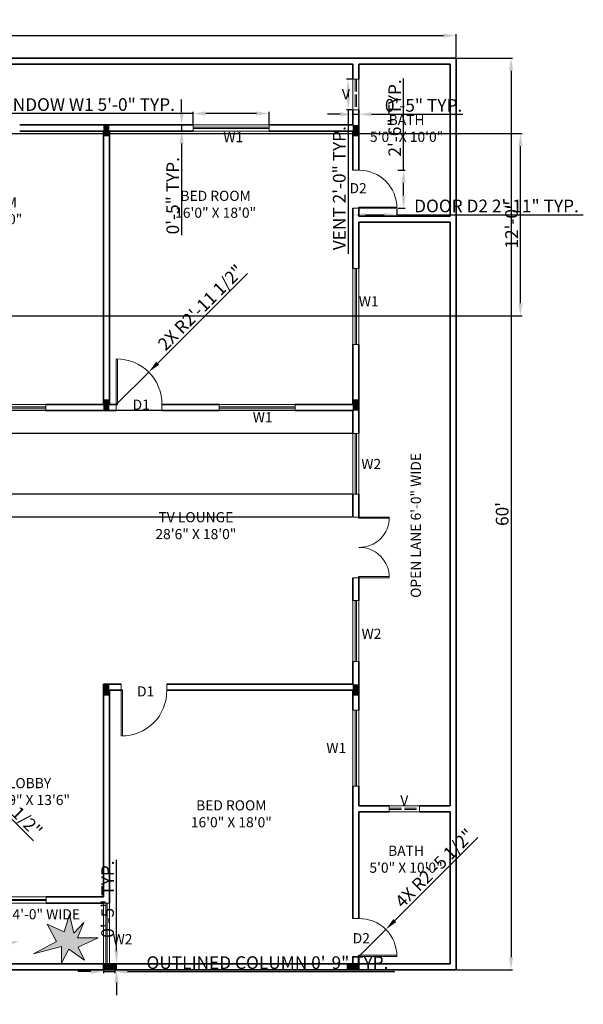
# Model space of a CAD drawing. Units: inches. Extents: x 13878 to 15021, y 3891 to 4810.
# Tile 3 of 3: x 14576 to 15021, y 3923 to 4701. Entities that reach past the tile are written whole.
import ezdxf

# ---------------------------------------------------------------- set-up
doc = ezdxf.new("R2010")
doc.units = ezdxf.units.IN
doc.linetypes.add('ACAD_ISO02W100', pattern=[15, 12, -3])
for name, color, linetype, lineweight in [('A-ANNO-DIMS', 2, 'Continuous', 18), ('A-ANNO-TEXT', 7, 'Continuous', 18), ('A-AREA-IDEN', 7, 'Continuous', 18), ('A-COLS', 7, 'Continuous', 35), ('A-COLS-PATT', 7, 'Continuous', 18), ('A-DOOR', 4, 'Continuous', 18), ('A-GLAZ', 4, 'Continuous', 18), ('A-GLAZ-HIDN', 4, 'ACAD_ISO02W100', 13), ('A-WALL', 150, 'Continuous', 35), ('C-SITE-WALL', 150, 'Continuous', 35), ('L-PLNT', 85, 'Continuous', 18)]:
    doc.layers.add(name, color=color, linetype=linetype, lineweight=lineweight)
doc.layers.add('L-PLNT-PATT', color=85, linetype='Continuous', lineweight=13, true_color=0x58ba48)
doc.styles.get("Standard").update_dxf_attribs({"font": 'arial.ttf'})
doc.dimstyles.new('ISO-25', dxfattribs={"dimtxt": 10, "dimasz": 10, "dimexe": 1.25, "dimexo": 0.625, "dimtad": 1, "dimdec": 0, "dimlunit": 3, "dimtxsty": 'Standard', "dimcen": 2.5, "dimadec": 0, "dimazin": 0, "dimtfac": 1, "dimtdec": 0, "dimtmove": 0, "dimatfit": 3, "dimfxl": 1, "dimarcsym": 0})

# ---------------------------------------------------------------- blocks, each defined once
blk = doc.blocks.new('*D7')
at = {"layer": 'A-ANNO-DIMS', "color": 0, "lineweight": -2, "transparency": 16777216}
for p, q in [((13960.64, 4671.28), (13960.64, 4689.65)), ((13970.64, 4688.4), (14910.64, 4688.4)), ((14920.64, 4671.28), (14920.64, 4689.65))]:
    blk.add_line(p, q, dxfattribs=at)
at = {"layer": 'A-ANNO-DIMS', "color": 0, "transparency": 16777216}
for points in [[(13970.64, 4690.07), (13970.64, 4686.74), (13960.64, 4688.4)], [(14910.64, 4690.07), (14910.64, 4686.74), (14920.64, 4688.4)]]:
    blk.add_solid(points, dxfattribs=at)
at = {"layer": 'Defpoints', "color": 0, "transparency": 16777216}
for p in [(14920.64, 4688.4), (13960.64, 4670.66), (14920.64, 4670.66)]:
    blk.add_point(p, dxfattribs=at)
at = {"layer": 'A-ANNO-DIMS', "color": 0, "transparency": 16777216, "insert": (14440.64, 4694.14), "char_height": 10, "attachment_point": 5}
blk.add_mtext("80'", dxfattribs=at)
blk = doc.blocks.new('*D8')
at = {"layer": 'A-ANNO-DIMS', "color": 0, "lineweight": -2, "transparency": 16777216}
for p, q in [((14921.26, 4670.66), (14965.22, 4670.66)), ((14963.97, 4660.66), (14963.97, 3960.66)), ((14921.26, 3950.66), (14965.22, 3950.66))]:
    blk.add_line(p, q, dxfattribs=at)
at = {"layer": 'A-ANNO-DIMS', "color": 0, "transparency": 16777216}
for points in [[(14962.31, 4660.66), (14965.64, 4660.66), (14963.97, 4670.66)], [(14962.31, 3960.66), (14965.64, 3960.66), (14963.97, 3950.66)]]:
    blk.add_solid(points, dxfattribs=at)
at = {"layer": 'Defpoints', "color": 0, "transparency": 16777216}
for p in [(14920.64, 4670.66), (14920.64, 3950.66), (14963.97, 3950.66)]:
    blk.add_point(p, dxfattribs=at)
at = {"layer": 'A-ANNO-DIMS', "color": 0, "transparency": 16777216, "insert": (14958.24, 4310.66), "char_height": 10, "attachment_point": 5, "rotation": 90}
blk.add_mtext("60'", dxfattribs=at)
blk = doc.blocks.new('DOOR-D1-36IN')
for p, q in [((0, 4.8), (0, 40.8)), ((1, 4.8), (1, 40.8)), ((0, 4.8), (0, 0)), ((36, 4.8), (36, 0))]:
    blk.add_line(p, q)
blk.add_arc((0.5, 5.3), 35.5, 359.19307, 90.80693)
blk = doc.blocks.new('DOOR-D2-30IN')
for p, q in [((0, 30), (4.8, 30)), ((0, 0), (4.8, 0)), ((4.8, 1), (34.8, 1)), ((4.8, 0), (34.8, 0))]:
    blk.add_line(p, q)
blk.add_arc((5.3, 0.5), 29.5, 359.02898, 90.97102)
blk = doc.blocks.new('DOOR-PAIR-48IN')
for p, q in [((0, 48), (4.8, 48)), ((4.8, 48), (28.8, 48)), ((4.8, 47), (28.8, 47)), ((4.8, 1), (28.8, 1)), ((0, 0), (4.8, 0)), ((4.8, 0), (28.8, 0))]:
    blk.add_line(p, q)
for centre, start, end in [((5.3, 47.5), 268.78112, 1.21888), ((5.3, 0.5), 358.78112, 91.21888)]:
    blk.add_arc(centre, 23.51, start, end)
blk = doc.blocks.new('WINDOW-W1-60IN')
for p, q in [((0, 0), (0, 4.8)), ((0, 4.8), (60, 4.8)), ((0, 2.9), (60, 2.9)), ((0, 1.9), (60, 1.9)), ((60, 0), (60, 4.8)), ((0, 0), (60, 0))]:
    blk.add_line(p, q)
blk = doc.blocks.new('WINDOW-W2-48IN')
for p, q in [((0, 0), (0, 4.8)), ((0, 4.8), (48, 4.8)), ((0, 2.9), (48, 2.9)), ((0, 1.9), (48, 1.9)), ((48, 0), (48, 4.8)), ((0, 0), (48, 0))]:
    blk.add_line(p, q)
blk = doc.blocks.new('COLUMN-RECT-OUTLINED')
h = blk.add_hatch(color=256)
h.dxf.hatch_style = 1
h.paths.add_polyline_path([(9, 0), (9, 4.8), (0, 4.8), (0, 0)])
for p, q in [((0, 4.8), (0, 0)), ((9, 4.8), (0, 4.8)), ((9, 0), (9, 4.8)), ((0, 0), (9, 0))]:
    blk.add_line(p, q)
blk = doc.blocks.new('COLUMN-RECT-SOLID')
h = blk.add_hatch(color=256)
h.dxf.hatch_style = 1
h.paths.add_polyline_path([(0, 0), (4.8, 0), (4.8, 9), (0, 9)])
blk = doc.blocks.new('VENT-FRAME-24IN')
for p, q in [((0, 0), (0, 4.8)), ((0, 4.8), (24, 4.8)), ((24, 0), (24, 4.8)), ((0, 0), (24, 0))]:
    blk.add_line(p, q)
blk = doc.blocks.new('*D20')
at = {"layer": 'A-ANNO-DIMS', "color": 0, "lineweight": -2, "ltscale": 2, "transparency": 16777216}
for p, q in [((14642.24, 3950.03), (14642.24, 3948.06)), ((14651.24, 3950.03), (14651.24, 3948.06)), ((14632.24, 3949.31), (14622.24, 3949.31)), ((14642.24, 3949.31), (14651.24, 3949.31)), ((14661.24, 3949.31), (14872.28, 3949.31))]:
    blk.add_line(p, q, dxfattribs=at)
at = {"layer": 'A-ANNO-DIMS', "color": 0, "ltscale": 2, "transparency": 16777216}
for points in [[(14632.24, 3950.98), (14632.24, 3947.64), (14642.24, 3949.31)], [(14661.24, 3950.98), (14661.24, 3947.64), (14651.24, 3949.31)]]:
    blk.add_solid(points, dxfattribs=at)
at = {"layer": 'Defpoints', "color": 0, "ltscale": 2, "transparency": 16777216}
for p in [(14642.24, 3950.66), (14651.24, 3950.66), (14651.24, 3949.31)]:
    blk.add_point(p, dxfattribs=at)
at = {"layer": 'A-ANNO-DIMS', "color": 0, "ltscale": 2, "transparency": 16777216, "insert": (14771.76, 3955.11), "char_height": 10, "attachment_point": 5}
blk.add_mtext('OUTLINED COLUMN 0\'-9" TYP.', dxfattribs=at)
blk = doc.blocks.new('*D21')
at = {"layer": 'A-ANNO-DIMS', "color": 0, "lineweight": -2, "ltscale": 2, "transparency": 16777216}
for p, q in [((14652.59, 3965.46), (14652.59, 4037.66)), ((14651.86, 3955.46), (14653.84, 3955.46)), ((14651.86, 3950.66), (14653.84, 3950.66)), ((14652.59, 3950.66), (14652.59, 3955.46)), ((14652.59, 3940.66), (14652.59, 3930.66))]:
    blk.add_line(p, q, dxfattribs=at)
at = {"layer": 'A-ANNO-DIMS', "color": 0, "ltscale": 2, "transparency": 16777216}
for points in [[(14650.92, 3965.46), (14654.25, 3965.46), (14652.59, 3955.46)], [(14650.92, 3940.66), (14654.25, 3940.66), (14652.59, 3950.66)]]:
    blk.add_solid(points, dxfattribs=at)
at = {"layer": 'Defpoints', "color": 0, "ltscale": 2, "transparency": 16777216}
for p in [(14651.24, 3955.46), (14651.24, 3950.66), (14652.59, 3955.46)]:
    blk.add_point(p, dxfattribs=at)
at = {"layer": 'A-ANNO-DIMS', "color": 0, "ltscale": 2, "transparency": 16777216, "insert": (14646.86, 4006.56), "char_height": 10, "attachment_point": 5, "rotation": 90}
blk.add_mtext('0\'-5" TYP.', dxfattribs=at)
blk = doc.blocks.new('*D24')
at = {"layer": 'A-ANNO-DIMS', "color": 0, "lineweight": -2, "ltscale": 2, "transparency": 16777216}
for p, q in [((14713.04, 4626.86), (14550.41, 4626.86)), ((14713.04, 4618.48), (14713.04, 4628.11)), ((14763.04, 4626.86), (14723.04, 4626.86)), ((14773.04, 4618.48), (14773.04, 4628.11))]:
    blk.add_line(p, q, dxfattribs=at)
at = {"layer": 'A-ANNO-DIMS', "color": 0, "ltscale": 2, "transparency": 16777216}
for points in [[(14723.04, 4628.53), (14723.04, 4625.19), (14713.04, 4626.86)], [(14763.04, 4628.53), (14763.04, 4625.19), (14773.04, 4626.86)]]:
    blk.add_solid(points, dxfattribs=at)
at = {"layer": 'Defpoints', "color": 0, "ltscale": 2, "transparency": 16777216}
for p in [(14713.04, 4626.86), (14713.04, 4617.86), (14773.04, 4617.86)]:
    blk.add_point(p, dxfattribs=at)
at = {"layer": 'A-ANNO-DIMS', "color": 0, "ltscale": 2, "transparency": 16777216, "insert": (14626.72, 4632.66), "char_height": 10, "attachment_point": 5}
blk.add_mtext('WINDOW W1 5\'-0" TYP.', dxfattribs=at)
blk = doc.blocks.new('*D25')
at = {"layer": 'A-ANNO-DIMS', "color": 0, "lineweight": -2, "ltscale": 2, "transparency": 16777216}
for p, q in [((14704.04, 4627.86), (14704.04, 4637.86)), ((14712.41, 4617.86), (14702.79, 4617.86)), ((14712.41, 4613.06), (14702.79, 4613.06)), ((14704.04, 4617.86), (14704.04, 4613.06)), ((14704.04, 4603.06), (14704.04, 4530.85))]:
    blk.add_line(p, q, dxfattribs=at)
at = {"layer": 'A-ANNO-DIMS', "color": 0, "ltscale": 2, "transparency": 16777216}
for points in [[(14702.37, 4627.86), (14705.7, 4627.86), (14704.04, 4617.86)], [(14702.37, 4603.06), (14705.7, 4603.06), (14704.04, 4613.06)]]:
    blk.add_solid(points, dxfattribs=at)
at = {"layer": 'Defpoints', "color": 0, "ltscale": 2, "transparency": 16777216}
for p in [(14704.04, 4613.06), (14713.04, 4617.86), (14713.04, 4613.06)]:
    blk.add_point(p, dxfattribs=at)
at = {"layer": 'A-ANNO-DIMS', "color": 0, "ltscale": 2, "transparency": 16777216, "insert": (14698.31, 4561.96), "char_height": 10, "attachment_point": 5, "rotation": 90}
blk.add_mtext('0\'-5" TYP.', dxfattribs=at)
blk = doc.blocks.new('*D28')
at = {"layer": 'A-ANNO-DIMS', "color": 0, "lineweight": -2, "ltscale": 2, "transparency": 16777216}
for p, q in [((14838.41, 4653.86), (14834.19, 4653.86)), ((14835.44, 4643.86), (14835.44, 4639.86)), ((14838.41, 4629.86), (14834.19, 4629.86)), ((14835.44, 4629.86), (14835.44, 4516))]:
    blk.add_line(p, q, dxfattribs=at)
at = {"layer": 'A-ANNO-DIMS', "color": 0, "ltscale": 2, "transparency": 16777216}
for points in [[(14833.77, 4643.86), (14837.1, 4643.86), (14835.44, 4653.86)], [(14833.77, 4639.86), (14837.1, 4639.86), (14835.44, 4629.86)]]:
    blk.add_solid(points, dxfattribs=at)
at = {"layer": 'Defpoints', "color": 0, "ltscale": 2, "transparency": 16777216}
for p in [(14839.04, 4653.86), (14835.44, 4629.86), (14839.04, 4629.86)]:
    blk.add_point(p, dxfattribs=at)
at = {"layer": 'A-ANNO-DIMS', "color": 0, "ltscale": 2, "transparency": 16777216, "insert": (14829.71, 4567.93), "char_height": 10, "attachment_point": 5, "rotation": 90}
blk.add_mtext('VENT 2\'-0" TYP.', dxfattribs=at)
blk = doc.blocks.new('*D29')
at = {"layer": 'A-ANNO-DIMS', "color": 0, "lineweight": -2, "ltscale": 2, "transparency": 16777216}
for p, q in [((14829.04, 4626.26), (14819.04, 4626.26)), ((14839.04, 4629.23), (14839.04, 4625.01)), ((14839.04, 4626.26), (14843.84, 4626.26)), ((14843.84, 4629.23), (14843.84, 4625.01)), ((14853.84, 4626.26), (14926.04, 4626.26))]:
    blk.add_line(p, q, dxfattribs=at)
at = {"layer": 'A-ANNO-DIMS', "color": 0, "ltscale": 2, "transparency": 16777216}
for points in [[(14829.04, 4627.93), (14829.04, 4624.59), (14839.04, 4626.26)], [(14853.84, 4627.93), (14853.84, 4624.59), (14843.84, 4626.26)]]:
    blk.add_solid(points, dxfattribs=at)
at = {"layer": 'Defpoints', "color": 0, "ltscale": 2, "transparency": 16777216}
for p in [(14839.04, 4629.86), (14843.84, 4629.86), (14843.84, 4626.26)]:
    blk.add_point(p, dxfattribs=at)
at = {"layer": 'A-ANNO-DIMS', "color": 0, "ltscale": 2, "transparency": 16777216, "insert": (14894.94, 4631.99), "char_height": 10, "attachment_point": 5}
blk.add_mtext('0\'-5" TYP.', dxfattribs=at)
blk = doc.blocks.new('*D32')
at = {"layer": 'A-ANNO-DIMS', "color": 0, "lineweight": -2, "ltscale": 2, "transparency": 16777216}
for p, q in [((14839.04, 4551.41), (14839.04, 4545.54)), ((14873.97, 4551.41), (14873.97, 4545.54)), ((14849.04, 4546.79), (14863.97, 4546.79)), ((14873.97, 4546.79), (15020.98, 4546.79))]:
    blk.add_line(p, q, dxfattribs=at)
at = {"layer": 'A-ANNO-DIMS', "color": 0, "ltscale": 2, "transparency": 16777216}
for points in [[(14849.04, 4548.46), (14849.04, 4545.13), (14839.04, 4546.79)], [(14863.97, 4548.46), (14863.97, 4545.13), (14873.97, 4546.79)]]:
    blk.add_solid(points, dxfattribs=at)
at = {"layer": 'Defpoints', "color": 0, "ltscale": 2, "transparency": 16777216}
for p in [(14839.04, 4552.03), (14873.97, 4552.03), (14873.97, 4546.79)]:
    blk.add_point(p, dxfattribs=at)
at = {"layer": 'A-ANNO-DIMS', "color": 0, "ltscale": 2, "transparency": 16777216, "insert": (14952.48, 4552.59), "char_height": 10, "attachment_point": 5}
blk.add_mtext('DOOR D2 2\'-11" TYP.', dxfattribs=at)
blk = doc.blocks.new('*D33')
at = {"layer": 'A-ANNO-DIMS', "color": 0, "lineweight": -2, "ltscale": 2, "transparency": 16777216}
for p, q in [((14879.21, 4582.17), (14879.21, 4654.54)), ((14874.6, 4582.17), (14880.46, 4582.17)), ((14879.21, 4562.03), (14879.21, 4572.17)), ((14874.6, 4552.03), (14880.46, 4552.03))]:
    blk.add_line(p, q, dxfattribs=at)
at = {"layer": 'A-ANNO-DIMS', "color": 0, "ltscale": 2, "transparency": 16777216}
for points in [[(14877.55, 4572.17), (14880.88, 4572.17), (14879.21, 4582.17)], [(14877.55, 4562.03), (14880.88, 4562.03), (14879.21, 4552.03)]]:
    blk.add_solid(points, dxfattribs=at)
at = {"layer": 'Defpoints', "color": 0, "ltscale": 2, "transparency": 16777216}
for p in [(14873.97, 4582.17), (14879.21, 4582.17), (14873.97, 4552.03)]:
    blk.add_point(p, dxfattribs=at)
at = {"layer": 'A-ANNO-DIMS', "color": 0, "ltscale": 2, "transparency": 16777216, "insert": (14873.48, 4623.36), "char_height": 10, "attachment_point": 5, "rotation": 90}
blk.add_mtext('2\'-6" TYP.', dxfattribs=at)
blk = doc.blocks.new('*D37')
at = {"layer": 'A-ANNO-DIMS', "color": 0, "lineweight": -2, "ltscale": 2, "transparency": 16777216}
for p, q in [((14030.86, 4611.06), (14972.64, 4611.06)), ((14971.39, 4477.06), (14971.39, 4601.06)), ((14030.86, 4467.06), (14972.64, 4467.06))]:
    blk.add_line(p, q, dxfattribs=at)
at = {"layer": 'A-ANNO-DIMS', "color": 0, "ltscale": 2, "transparency": 16777216}
for points in [[(14969.72, 4601.06), (14973.05, 4601.06), (14971.39, 4611.06)], [(14969.72, 4477.06), (14973.05, 4477.06), (14971.39, 4467.06)]]:
    blk.add_solid(points, dxfattribs=at)
at = {"layer": 'Defpoints', "color": 0, "ltscale": 2, "transparency": 16777216}
for p in [(14030.24, 4611.06), (14971.39, 4611.06), (14030.24, 4467.06)]:
    blk.add_point(p, dxfattribs=at)
at = {"layer": 'A-ANNO-DIMS', "color": 0, "ltscale": 2, "transparency": 16777216, "insert": (14965.66, 4539.06), "char_height": 10, "attachment_point": 5, "rotation": 90}
blk.add_mtext('12\'-0"', dxfattribs=at)
blk = doc.blocks.new('*D40')
at = {"layer": 'A-ANNO-DIMS', "color": 0, "lineweight": -2, "ltscale": 2, "transparency": 16777216}
for p, q in [((13909.89, 4402.26), (13909.89, 4412.26)), ((14838.41, 4392.26), (13908.64, 4392.26)), ((13909.89, 4392.26), (13909.89, 4374.26)), ((14838.41, 4374.26), (13908.64, 4374.26)), ((13909.89, 4364.26), (13909.89, 4327.37))]:
    blk.add_line(p, q, dxfattribs=at)
at = {"layer": 'A-ANNO-DIMS', "color": 0, "ltscale": 2, "transparency": 16777216}
for points in [[(13908.22, 4402.26), (13911.55, 4402.26), (13909.89, 4392.26)], [(13908.22, 4364.26), (13911.55, 4364.26), (13909.89, 4374.26)]]:
    blk.add_solid(points, dxfattribs=at)
at = {"layer": 'Defpoints', "color": 0, "ltscale": 2, "transparency": 16777216}
for p in [(14839.04, 4392.26), (13909.89, 4374.26), (14839.04, 4374.26)]:
    blk.add_point(p, dxfattribs=at)
at = {"layer": 'A-ANNO-DIMS', "color": 0, "ltscale": 2, "transparency": 16777216, "insert": (13904.16, 4340.81), "char_height": 10, "attachment_point": 5, "rotation": 90}
blk.add_mtext('1\'-6"', dxfattribs=at)
blk = doc.blocks.new('*D41')
at = {"layer": 'A-ANNO-DIMS', "color": 0, "lineweight": -2, "ltscale": 2, "transparency": 16777216}
for p, q in [((13909.89, 4336.26), (13909.89, 4346.26)), ((14838.41, 4326.26), (13908.64, 4326.26)), ((13909.89, 4326.26), (13909.89, 4308.26)), ((14838.41, 4308.26), (13908.64, 4308.26)), ((13909.89, 4298.26), (13909.89, 4261.37))]:
    blk.add_line(p, q, dxfattribs=at)
at = {"layer": 'A-ANNO-DIMS', "color": 0, "ltscale": 2, "transparency": 16777216}
for points in [[(13908.22, 4336.26), (13911.55, 4336.26), (13909.89, 4326.26)], [(13908.22, 4298.26), (13911.55, 4298.26), (13909.89, 4308.26)]]:
    blk.add_solid(points, dxfattribs=at)
at = {"layer": 'Defpoints', "color": 0, "ltscale": 2, "transparency": 16777216}
for p in [(14839.04, 4326.26), (13909.89, 4308.26), (14839.04, 4308.26)]:
    blk.add_point(p, dxfattribs=at)
at = {"layer": 'A-ANNO-DIMS', "color": 0, "ltscale": 2, "transparency": 16777216, "insert": (13904.16, 4274.81), "char_height": 10, "attachment_point": 5, "rotation": 90}
blk.add_mtext('1\'-6"', dxfattribs=at)
blk = doc.blocks.new('*D48')
at = {"layer": 'A-ANNO-DIMS', "color": 0, "lineweight": -2, "ltscale": 2, "transparency": 16777216}
for p, q in [((14755.92, 4500.54), (14685.12, 4429.74)), ((14652.94, 4397.56), (14678.05, 4422.66))]:
    blk.add_line(p, q, dxfattribs=at)
at = {"layer": 'A-ANNO-DIMS', "color": 0, "ltscale": 2, "transparency": 16777216}
blk.add_solid([(14683.94, 4430.91), (14686.3, 4428.56), (14678.05, 4422.66)], dxfattribs=at)
at = {"layer": 'Defpoints', "color": 0, "ltscale": 2, "transparency": 16777216}
for p in [(14678.05, 4422.66), (14652.94, 4397.56)]:
    blk.add_point(p, dxfattribs=at)
at = {"layer": 'A-ANNO-DIMS', "color": 0, "ltscale": 2, "transparency": 16777216, "insert": (14719.96, 4472.77), "char_height": 10, "attachment_point": 5, "rotation": 45.00017}
blk.add_mtext('2X R2\'-11 1/2"', dxfattribs=at)
blk = doc.blocks.new('*D49')
at = {"layer": 'A-ANNO-DIMS', "color": 0, "lineweight": -2, "ltscale": 2, "transparency": 16777216}
for p, q in [((14937.75, 4055.12), (14872.27, 3989.65)), ((14844.34, 3961.71), (14865.2, 3982.58))]:
    blk.add_line(p, q, dxfattribs=at)
at = {"layer": 'A-ANNO-DIMS', "color": 0, "ltscale": 2, "transparency": 16777216}
blk.add_solid([(14871.09, 3990.83), (14873.45, 3988.47), (14865.2, 3982.58)], dxfattribs=at)
at = {"layer": 'Defpoints', "color": 0, "ltscale": 2, "transparency": 16777216}
for p in [(14865.2, 3982.58), (14844.34, 3961.71)]:
    blk.add_point(p, dxfattribs=at)
at = {"layer": 'A-ANNO-DIMS', "color": 0, "ltscale": 2, "transparency": 16777216, "insert": (14904.45, 4030.02), "char_height": 10, "attachment_point": 5, "rotation": 44.99985}
blk.add_mtext('4X R2\'-5 1/2"', dxfattribs=at)
blk = doc.blocks.new('*D50')
at = {"layer": 'A-ANNO-DIMS', "color": 0, "lineweight": -2, "ltscale": 2, "transparency": 16777216}
for p, q in [((14492.74, 4146.96), (14509.36, 4130.34)), ((14587.15, 4052.55), (14516.43, 4123.27))]:
    blk.add_line(p, q, dxfattribs=at)
at = {"layer": 'A-ANNO-DIMS', "color": 0, "ltscale": 2, "transparency": 16777216}
blk.add_solid([(14517.61, 4124.45), (14515.25, 4122.09), (14509.36, 4130.34)], dxfattribs=at)
at = {"layer": 'Defpoints', "color": 0, "ltscale": 2, "transparency": 16777216}
for p in [(14492.74, 4146.96), (14509.36, 4130.34)]:
    blk.add_point(p, dxfattribs=at)
at = {"layer": 'A-ANNO-DIMS', "color": 0, "ltscale": 2, "transparency": 16777216, "insert": (14559.42, 4088.47), "char_height": 10, "attachment_point": 5, "rotation": 315.00023}
blk.add_mtext('6X R1\'-11 1/2"', dxfattribs=at)

msp = doc.modelspace()

# ---------------------------------------------------------------- hatches: boundary and pattern name
at = {"layer": 'L-PLNT-PATT'}
h = msp.add_hatch(color=256, dxfattribs=at)
h.dxf.hatch_style = 1
h.paths.add_polyline_path([(14211.42, 4164.09), (14225.1, 4154.41), (14219.69, 4165.88), (14237.21, 4174.14), (14219.04, 4174.14), (14224.72, 4187.59), (14215.8, 4178.36), (14211.91, 4194.56), (14207.36, 4179.33), (14192.4, 4186.2), (14200.72, 4170.9), (14180.44, 4159.88), (14204.93, 4166.36), (14204.93, 4151.94)])
h.paths.add_polyline_path([(14260.1, 4167.9), (14271.74, 4159.67), (14267.14, 4169.42), (14282.03, 4176.45), (14266.58, 4176.45), (14271.41, 4187.89), (14263.83, 4180.03), (14260.52, 4193.82), (14256.65, 4180.86), (14243.93, 4186.7), (14251, 4173.69), (14233.76, 4164.32), (14254.58, 4169.83), (14254.58, 4157.57)])
h.paths.add_polyline_path([(14365.73, 4178.36), (14361.84, 4194.56), (14357.3, 4179.33), (14342.33, 4186.2), (14350.65, 4170.9), (14331.44, 4160.46), (14331.44, 4160.16), (14354.86, 4166.36), (14354.86, 4151.94), (14361.35, 4164.09), (14375.03, 4154.41), (14369.62, 4165.88), (14387.14, 4174.14), (14368.97, 4174.14), (14374.65, 4187.59)])
h.paths.add_polyline_path([(14420, 4174.14), (14425.67, 4187.59), (14416.75, 4178.36), (14412.86, 4194.56), (14408.32, 4179.33), (14393.35, 4186.2), (14401.67, 4170.9), (14381.4, 4159.88), (14405.89, 4166.36), (14405.89, 4151.94), (14412.37, 4164.09), (14426.05, 4154.41), (14420.65, 4165.88), (14438.16, 4174.14)])
h.paths.add_polyline_path([(14249.25, 4019.93), (14249.25, 4005.5), (14255.74, 4017.66), (14269.42, 4007.98), (14264.01, 4019.44), (14281.52, 4027.71), (14263.36, 4027.71), (14269.03, 4041.16), (14260.11, 4031.92), (14256.22, 4048.13), (14251.68, 4032.89), (14236.72, 4039.77), (14245.03, 4024.47), (14224.76, 4013.45)])
h.paths.add_polyline_path([(14203.49, 4032.89), (14188.53, 4039.77), (14196.84, 4024.47), (14176.57, 4013.45), (14201.06, 4019.93), (14201.06, 4005.5), (14207.55, 4017.66), (14221.23, 4007.98), (14215.82, 4019.44), (14233.33, 4027.71), (14215.17, 4027.71), (14220.85, 4041.16), (14211.93, 4031.92), (14208.03, 4048.13)])
h.paths.add_polyline_path([(14362.82, 4016.2), (14376.5, 4006.52), (14371.09, 4017.98), (14388.61, 4026.25), (14370.44, 4026.25), (14376.12, 4039.7), (14367.2, 4030.46), (14363.31, 4046.67), (14358.76, 4031.44), (14343.8, 4038.31), (14352.12, 4023.01), (14331.84, 4011.99), (14356.33, 4018.47), (14356.33, 4004.05)])
h.paths.add_polyline_path([(14408.41, 4030.85), (14393.45, 4037.72), (14401.76, 4022.42), (14381.49, 4011.4), (14405.98, 4017.88), (14405.98, 4003.46), (14412.47, 4015.62), (14426.15, 4005.94), (14420.74, 4017.4), (14438.25, 4025.66), (14420.09, 4025.66), (14425.77, 4039.12), (14416.85, 4029.88), (14412.95, 4046.08)])
h.paths.add_polyline_path([(14502.95, 3976.33), (14500.16, 3987.92), (14496.92, 3977.03), (14486.21, 3981.94), (14492.16, 3971), (14477.66, 3963.12), (14495.18, 3967.76), (14495.18, 3957.44), (14499.81, 3966.13), (14509.6, 3959.21), (14505.73, 3967.41), (14518.25, 3973.32), (14505.27, 3973.32), (14509.32, 3982.94)])
h.paths.add_polyline_path([(14552.74, 3977.57), (14541.18, 3982.88), (14547.61, 3971.06), (14531.95, 3962.55), (14550.86, 3967.56), (14550.86, 3956.41), (14555.87, 3965.8), (14566.44, 3958.33), (14562.26, 3967.18), (14575.79, 3973.56), (14561.76, 3973.56), (14566.15, 3983.95), (14559.26, 3976.82), (14556.25, 3989.34)])
h.paths.add_polyline_path([(14605.39, 3973.1), (14587.22, 3963.23), (14609.17, 3969.04), (14609.17, 3956.11), (14614.98, 3967), (14627.25, 3958.33), (14622.4, 3968.6), (14638.1, 3976.01), (14621.82, 3976.01), (14626.9, 3988.07), (14618.91, 3979.79), (14615.42, 3994.31), (14611.35, 3980.66), (14597.94, 3986.82)])

# ---------------------------------------------------------------- linework, layer by layer
at = {"layer": 'A-GLAZ'}
for p, q in [((14642.24, 4003.46), (14642.24, 3955.46)), ((14642.24, 4003.46), (14647.04, 4003.46)), ((14644.14, 4003.46), (14644.14, 3955.46)), ((14645.14, 4003.46), (14645.14, 3955.46)), ((14647.04, 4003.46), (14647.04, 3955.46))]:
    msp.add_line(p, q, dxfattribs=at)
at = {"layer": 'A-GLAZ-HIDN', "ltscale": 0.8}
for p, q in [((14840.94, 4653.86), (14840.94, 4629.86)), ((14841.94, 4653.86), (14841.94, 4629.86)), ((14867.84, 4078.36), (14891.84, 4078.36)), ((14867.84, 4077.36), (14891.84, 4077.36))]:
    msp.add_line(p, q, dxfattribs=at)
at = {"layer": 'A-WALL'}
for p, q in [((14839.04, 4665.86), (14839.04, 4653.86)), ((14843.84, 4665.86), (14843.84, 4653.86)), ((14839.04, 4629.86), (14839.04, 4617.86)), ((14843.84, 4629.86), (14843.84, 4582.03)), ((14576.24, 4617.86), (14713.04, 4617.86)), ((14576.24, 4613.06), (14642.24, 4613.06)), ((14642.24, 4613.06), (14642.24, 4397.06)), ((14647.04, 4613.06), (14647.04, 4397.06)), ((14647.04, 4613.06), (14713.04, 4613.06)), ((14773.04, 4617.86), (14839.04, 4617.86)), ((14773.04, 4613.06), (14839.04, 4613.06)), ((14839.04, 4613.06), (14839.04, 4582.03)), ((14839.04, 4552.03), (14839.04, 4504.55)), ((14843.84, 4553.03), (14843.84, 4545.86)), ((14843.84, 4545.86), (14915.84, 4545.86)), ((14843.84, 4541.06), (14915.84, 4541.06)), ((14843.84, 4541.06), (14843.84, 4504.55)), ((14839.04, 4444.55), (14839.04, 4397.06)), ((14843.84, 4444.55), (14843.84, 4374.26)), ((14596.91, 4397.06), (14642.24, 4397.06)), ((14647.04, 4397.06), (14653.44, 4397.06)), ((14688.44, 4397.06), (14733.74, 4397.06)), ((14793.74, 4397.06), (14839.04, 4397.06)), ((14596.91, 4392.26), (14642.24, 4392.26)), ((14642.24, 4392.26), (14652.44, 4392.26)), ((14688.44, 4392.26), (14733.74, 4392.26)), ((14793.74, 4392.26), (14839.04, 4392.26)), ((14839.04, 4392.26), (14839.04, 4374.26)), ((14839.04, 4326.26), (14839.04, 4308.26)), ((14843.84, 4326.26), (14843.84, 4307.26)), ((14843.84, 4261.26), (14843.84, 4242.26)), ((14839.04, 4260.26), (14839.04, 4242.26)), ((14839.04, 4194.26), (14839.04, 4176.26)), ((14843.84, 4194.26), (14843.84, 4155.86)), ((14642.24, 4176.26), (14642.24, 4008.26)), ((14656.32, 4176.26), (14642.24, 4176.26)), ((14839.04, 4176.26), (14692.32, 4176.26)), ((14647.04, 4171.46), (14647.04, 4003.46)), ((14657.32, 4171.46), (14647.04, 4171.46)), ((14839.04, 4171.46), (14692.32, 4171.46)), ((14839.04, 4171.46), (14839.04, 4155.86)), ((14839.04, 4095.86), (14839.04, 4080.26)), ((14843.84, 4095.86), (14843.84, 4080.26)), ((14839.04, 4080.26), (14839.04, 3991.21)), ((14867.84, 4080.26), (14843.84, 4080.26)), ((14843.84, 4075.46), (14843.84, 3991.21)), ((14867.84, 4075.46), (14843.84, 4075.46)), ((14915.84, 4080.26), (14891.84, 4080.26)), ((14915.84, 4075.46), (14891.84, 4075.46)), ((14642.24, 4008.26), (14597.24, 4008.26)), ((14642.24, 4003.46), (14597.24, 4003.46)), ((14839.04, 3961.21), (14839.04, 3955.46)), ((14843.84, 3962.21), (14843.84, 3955.46))]:
    msp.add_line(p, q, dxfattribs=at)
at = {"layer": 'C-SITE-WALL'}
for p, q in [((13960.64, 4670.66), (14920.64, 4670.66)), ((13965.44, 4665.86), (14839.04, 4665.86)), ((14843.84, 4665.86), (14915.84, 4665.86)), ((14915.84, 4665.86), (14915.84, 4545.86)), ((14920.64, 4670.66), (14920.64, 3950.66)), ((14915.84, 4541.06), (14915.84, 4080.26)), ((14915.84, 4075.46), (14915.84, 3955.46)), ((14920.64, 3950.66), (14176.41, 3950.66)), ((14642.24, 3955.46), (14487.44, 3955.46)), ((14839.04, 3955.46), (14647.04, 3955.46)), ((14915.84, 3955.46), (14843.84, 3955.46))]:
    msp.add_line(p, q, dxfattribs=at)
at = {"layer": 'L-PLNT'}
for p, q in [((14611.35, 3980.66), (14615.42, 3994.31)), ((14615.42, 3994.31), (14618.91, 3979.79)), ((14605.39, 3973.1), (14597.94, 3986.82)), ((14597.94, 3986.82), (14611.35, 3980.66)), ((14618.91, 3979.79), (14626.9, 3988.07)), ((14626.9, 3988.07), (14621.82, 3976.01)), ((14587.22, 3963.23), (14605.39, 3973.1)), ((14621.82, 3976.01), (14638.1, 3976.01)), ((14638.1, 3976.01), (14622.4, 3968.6)), ((14609.17, 3969.04), (14587.22, 3963.23)), ((14609.17, 3956.11), (14609.17, 3969.04)), ((14614.98, 3967), (14609.17, 3956.11)), ((14627.25, 3958.33), (14614.98, 3967)), ((14622.4, 3968.6), (14627.25, 3958.33))]:
    msp.add_line(p, q, dxfattribs=at)

# ---------------------------------------------------------------- block references
at = {"layer": 'A-COLS'}
for p in [(14642.24, 3950.66), (14834.84, 3950.66)]:
    msp.add_blockref('COLUMN-RECT-OUTLINED', p, dxfattribs=at)
at = {"layer": 'A-COLS-PATT'}
for p in [(14642.24, 4608.86), (14839.04, 4608.86), (14642.24, 4392.26), (14839.04, 4392.26), (14642.24, 4167.23), (14839.04, 4167.23)]:
    msp.add_blockref('COLUMN-RECT-SOLID', p, dxfattribs=at)
at = {"layer": 'A-DOOR'}
for name, p in [('DOOR-D2-30IN', (14839.04, 4552.03)), ('DOOR-D1-36IN', (14652.44, 4392.26)), ('DOOR-PAIR-48IN', (14839.04, 4260.26)), ('DOOR-D2-30IN', (14839.04, 3961.21))]:
    msp.add_blockref(name, p, dxfattribs=at)
at = {"layer": 'A-DOOR', "extrusion": (0, 0, -1), "zscale": -1, "rotation": 180}
msp.add_blockref('DOOR-D1-36IN', (-14656.32, 4176.26), dxfattribs=at)
at = {"layer": 'A-GLAZ'}
for name, p, rotation in [('VENT-FRAME-24IN', (14839.04, 4653.86), 270.0000000000008), ('WINDOW-W1-60IN', (14773.04, 4617.86), 180), ('WINDOW-W1-60IN', (14843.84, 4444.55), 89.99999999999662), ('WINDOW-W1-60IN', (14596.91, 4397.06), 180), ('WINDOW-W1-60IN', (14793.74, 4397.06), 180), ('WINDOW-W2-48IN', (14839.04, 4374.26), 270.0000000000116), ('WINDOW-W2-48IN', (14843.84, 4194.26), 89.99999999998582), ('WINDOW-W1-60IN', (14843.84, 4095.86), 89.99999999998626), ('VENT-FRAME-24IN', (14891.84, 4080.26), 180), ('WINDOW-W1-60IN', (14597.24, 4008.26), 180)]:
    msp.add_blockref(name, p, dxfattribs=dict(at, rotation=rotation))

# ---------------------------------------------------------------- texts
at = {"layer": 'A-ANNO-TEXT', "char_height": 8, "attachment_point": 1}
for s, insert in [('V', (14830.48, 4646.19)), ('W1', (14736.94, 4612.22)), ('D2', (14836.5, 4571.88)), ('W1', (14843.84, 4482.58)), ('D1', (14665.32, 4400.98)), ('W1', (14760.18, 4391.08)), ('W2', (14845.8, 4354.12)), ('W2', (14846.02, 4220.07)), ('D1', (14668.86, 4174.57)), ('W1', (14818.23, 4129.86)), ('V', (14876.6, 4088.48)), ('W2', (14649.56, 3978.91)), ('D2', (14839.03, 3979.68))]:
    msp.add_mtext_dynamic_manual_height_columns(s, width=16.3853, gutter_width=12.5, heights=[0], dxfattribs=dict(at, insert=insert))
at = {"layer": 'A-AREA-IDEN', "char_height": 8, "attachment_point": 1}
for s, width, insert in [('\\pxqc;BATH\\P5\'0" X 10\'0"', 60, (14851.55, 4625.82)), ('\\pxqc;BED ROOM\\P16\'0" X 18\'0"', 65.572, (14698.07, 4565.87)), ('\\pxqc;BED ROOM\\P16\'0" X 18\'0"', 65.572, (14513.52, 4560.81)), ('\\pxqc;TV LOUNGE\\P28\'6" X 18\'0"', 129.4248, (14650.56, 4312.12)), ('\\pxqc;LOBBY\\P12\'0" X 13\'6"', 129.4248, (14519.29, 4102.16)), ('\\pxqc;BED ROOM\\P16\'0" X 18\'0"', 65.572, (14710.44, 4084.58)), ('\\pxqc;BATH\\P5\'0" X 10\'0"', 60, (14851.11, 4048.71)), ('OPEN LANE 4\'-0" WIDE', 379.1288, (14509.45, 3998.61))]:
    msp.add_mtext_dynamic_manual_height_columns(s, width=width, gutter_width=12.5, heights=[0], dxfattribs=dict(at, insert=insert))
at = {"layer": 'A-AREA-IDEN', "insert": (14884.82, 4244.43), "char_height": 8, "attachment_point": 1, "rotation": 90}
msp.add_mtext_dynamic_manual_height_columns('OPEN LANE 6\'-0" WIDE', width=379.1288, gutter_width=12.5, heights=[0], dxfattribs=at)

# ---------------------------------------------------------------- dimensions: what is measured, and where the dimension line sits
at = {"layer": 'A-ANNO-DIMS'}
dim = msp.add_linear_dim(base=(14920.64, 4688.4), p1=(13960.64, 4670.66), p2=(14920.64, 4670.66), dimstyle='ISO-25', override={"dimclrd": 0, "dimclre": 0, "dimclrt": 0}, dxfattribs=at)
dim.commit()
dim.dimension.update_dxf_attribs({"geometry": '*D7', "text_midpoint": (14440.64, 4694.14)})
dim = msp.add_linear_dim(base=(14963.97, 3950.66), p1=(14920.64, 4670.66), p2=(14920.64, 3950.66), angle=90, dimstyle='ISO-25', override={"dimclrd": 0, "dimclre": 0, "dimclrt": 0}, dxfattribs=at)
dim.commit()
dim.dimension.update_dxf_attribs({"geometry": '*D8', "text_midpoint": (14958.24, 4310.66)})
at = {"layer": 'A-ANNO-DIMS', "ltscale": 2}
for base, p1, p2, angle, text, picture, middle in [((14713.04, 4626.86), (14773.04, 4617.86), (14713.04, 4617.86), 180, 'WINDOW W1 <> TYP.', '*D24', (14626.72, 4632.66)), ((14835.44, 4629.86), (14839.04, 4653.86), (14839.04, 4629.86), 270, 'VENT <> TYP.', '*D28', (14829.71, 4567.93)), ((14879.21, 4582.17), (14873.97, 4552.03), (14873.97, 4582.17), 90, '<> TYP.', '*D33', (14873.48, 4623.36)), ((14704.04, 4613.06), (14713.04, 4617.86), (14713.04, 4613.06), 270, '<> TYP.', '*D25', (14698.31, 4561.96)), ((14652.59, 3955.46), (14651.24, 3950.66), (14651.24, 3955.46), 90, '<> TYP.', '*D21', (14646.86, 4006.56))]:
    dim = msp.add_linear_dim(base=base, p1=p1, p2=p2, angle=angle, text=text, dimstyle='ISO-25', override={"dimdec": 1, "dimlfac": 1, "dimrnd": 0, "dimzin": 1, "dimdsep": 46, "dimlunit": 4, "dimfrac": 2}, dxfattribs=at)
    dim.commit()
    dim.dimension.update_dxf_attribs({"geometry": picture, "text_midpoint": middle})
for base, p1, p2, text, picture, middle in [((14843.84, 4626.26), (14839.04, 4629.86), (14843.84, 4629.86), '<> TYP.', '*D29', (14894.94, 4631.99)), ((14873.97, 4546.79), (14839.04, 4552.03), (14873.97, 4552.03), 'DOOR D2 <> TYP.', '*D32', (14952.48, 4552.59)), ((14651.24, 3949.31), (14642.24, 3950.66), (14651.24, 3950.66), 'OUTLINED COLUMN <> TYP.', '*D20', (14771.76, 3955.11))]:
    dim = msp.add_linear_dim(base=base, p1=p1, p2=p2, text=text, dimstyle='ISO-25', override={"dimdec": 1, "dimlfac": 1, "dimrnd": 0, "dimzin": 1, "dimdsep": 46, "dimlunit": 4, "dimfrac": 2}, dxfattribs=at)
    dim.commit()
    dim.dimension.update_dxf_attribs({"geometry": picture, "text_midpoint": middle})
for base, p1, p2, picture, middle in [((14971.39, 4611.06), (14030.24, 4467.06), (14030.24, 4611.06), '*D37', (14965.66, 4539.06)), ((13909.89, 4374.26), (14839.04, 4392.26), (14839.04, 4374.26), '*D40', (13904.16, 4340.81)), ((13909.89, 4308.26), (14839.04, 4326.26), (14839.04, 4308.26), '*D41', (13904.16, 4274.81))]:
    dim = msp.add_linear_dim(base=base, p1=p1, p2=p2, angle=90, dimstyle='ISO-25', override={"dimdec": 1, "dimlfac": 1, "dimrnd": 0, "dimzin": 1, "dimdsep": 46, "dimlunit": 4, "dimfrac": 2}, dxfattribs=at)
    dim.commit()
    dim.dimension.update_dxf_attribs({"geometry": picture, "text_midpoint": middle})
for center, mpoint, text, picture, middle in [((14652.94, 4397.56), (14678.05, 4422.66), '2X <>', '*D48', (14719.96, 4472.77)), ((14492.74, 4146.96), (14509.36, 4130.34), '6X <>', '*D50', (14559.42, 4088.47)), ((14844.34, 3961.71), (14865.2, 3982.58), '4X <>', '*D49', (14904.45, 4030.02))]:
    dim = msp.add_radius_dim(center=center, mpoint=mpoint, text=text, dimstyle='ISO-25', override={"dimdec": 1, "dimlfac": 1, "dimrnd": 0, "dimzin": 1, "dimdsep": 46, "dimlunit": 4, "dimfrac": 2}, dxfattribs=at)
    dim.commit()
    dim.dimension.update_dxf_attribs({"geometry": picture, "text_midpoint": middle})

doc.saveas('drawing.dxf')
